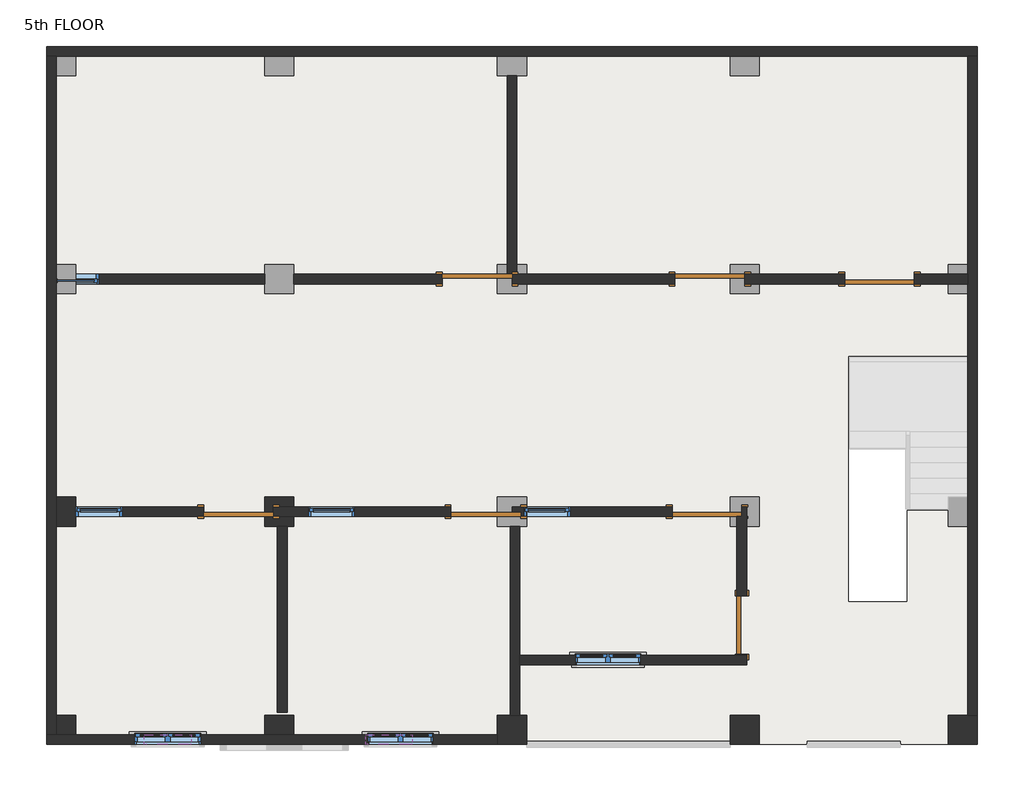
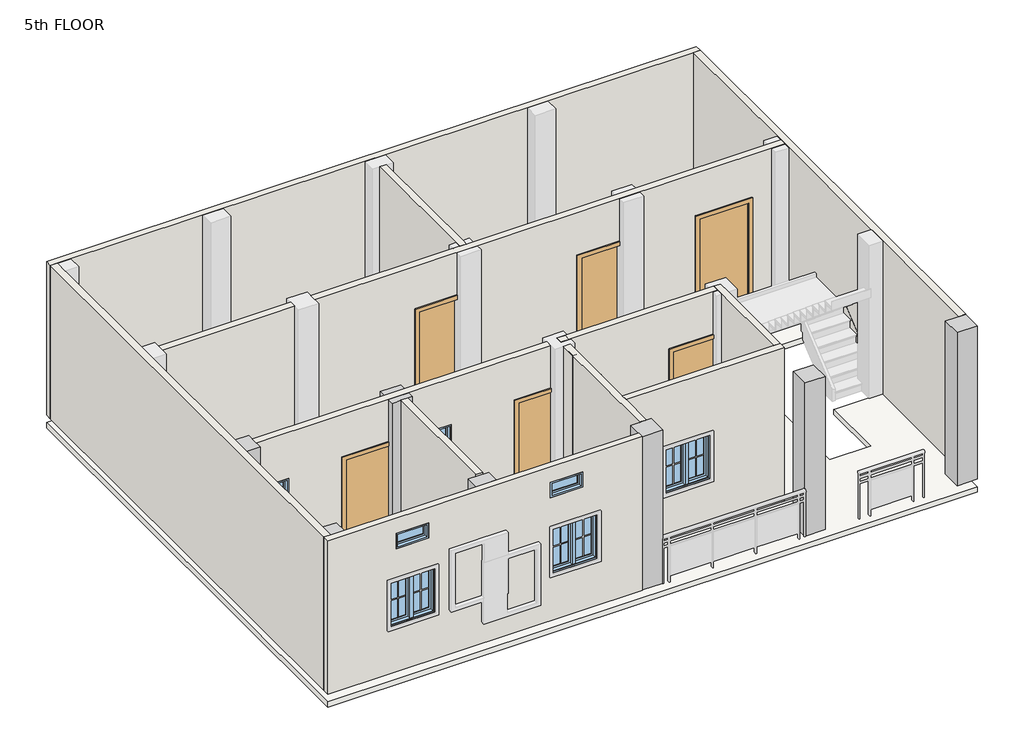
# One storey, part 1 of 2: 15 walls, 9 windows, 7 columns, 7 doors, 1 slab.
"""IFC4 building model written with IfcOpenShell, lengths in millimetres."""

from ifc_helpers import new_model, si_unit, frame, origin, place, context, project, spatial, polyline, outline, extrude, faceted_brep, transform, mapped, element, save
from components import door_e00f436c, door_a1797ceb, window_4c2727af, window_0bf3737e, window_78893e6c, window_0d9958e7

model = new_model("IFC4")

# Units and contexts
model_context = context("Model", 3, world=origin())
ifc_project = project(units=[si_unit("LENGTHUNIT", "METRE", prefix="MILLI")], contexts=[model_context])

# Site, building, storey
site = spatial("IfcSite", under=ifc_project)
building = spatial("IfcBuilding", under=site)
storey = spatial("IfcBuildingStorey", under=building, Name="5th FLOOR", Elevation=15087.6)

# Columns
placement = place(None, origin())
element("IfcColumn", 1, ObjectType="column family : column family", at=placement, inside=storey, context=model_context, shape_type="Brep", body=[
    faceted_brep([(-12576.097125, 2486.2065522, 15092.6), (-12957.097125, 2486.2065522, 15092.6), (-12957.097125, 2867.2065522, 15092.6), (-12576.097125, 2867.2065522, 15092.6), (-12576.097125, 2740.2065522, 15092.6), (-12842.797125, 2740.2065522, 15092.6), (-12842.797125, 2613.2065522, 15092.6), (-12576.097125, 2613.2065522, 15092.6), (-12576.097125, 2486.2065522, 18130.6), (-12576.097125, 2613.2065522, 18130.6), (-12957.097125, 2486.2065522, 18130.6), (-12957.097125, 2613.2065522, 18130.6), (-12957.097125, 2613.2065522, 17221.2), (-12957.097125, 2740.2065522, 17221.2), (-12957.097125, 2740.2065522, 18130.6), (-12957.097125, 2867.2065522, 18130.6), (-12576.097125, 2867.2065522, 18130.6), (-12842.797125, 2613.2065522, 17221.2), (-12842.797125, 2740.2065522, 17221.2), (-12576.097125, 2740.2065522, 18130.6)], [[[0, 1, 2, 3, 4, 5, 6, 7]], [[8, 0, 7, 9]], [[1, 0, 8, 10]], [[2, 1, 10, 11, 12, 13, 14, 15]], [[3, 2, 15, 16]], [[10, 8, 9, 11]], [[6, 17, 12, 11, 9, 7]], [[13, 18, 5, 4, 19, 14]], [[3, 16, 19, 4]], [[16, 15, 14, 19]], [[17, 18, 13, 12]], [[18, 17, 6, 5]]]),
])
element("IfcColumn", 2, ObjectType="column family : column family", at=placement, inside=storey, context=model_context, shape_type="SweptSolid", body=[
    extrude(outline(polyline([(-15433.597125, 2867.2065522), (-15433.597125, 2486.2065522), (-15687.597125, 2486.2065522), (-15687.597125, 2867.2065522), (-15433.597125, 2867.2065522)])), frame((0.0, 0.0, 15092.6), z_axis=(0.0, 0.0, 1.0), x_axis=(1.0, 0.0, 0.0)), (0.0, 0.0, 1.0), 3038.0),
])
element("IfcColumn", 3, ObjectType="column family : column family", at=placement, inside=storey, context=model_context, shape_type="SweptSolid", body=[
    extrude(outline(polyline([(-15433.597125, 9.7065522), (-15433.597125, -244.2934478), (-15687.597125, -244.2934478), (-15687.597125, 9.7065522), (-15433.597125, 9.7065522)])), frame((0.0, 0.0, 15092.6), z_axis=(0.0, 0.0, 1.0), x_axis=(1.0, 0.0, 0.0)), (0.0, 0.0, 1.0), 3038.0),
])
element("IfcColumn", 4, ObjectType="column family : column family", at=placement, inside=storey, context=model_context, shape_type="SweptSolid", body=[
    extrude(outline(polyline([(-3622.597125, 9.7065522), (-3622.597125, -371.2934478), (-4003.597125, -371.2934478), (-4003.597125, 9.7065522), (-3622.597125, 9.7065522)])), frame((0.0, 0.0, 15092.6), z_axis=(0.0, 0.0, 1.0), x_axis=(1.0, 0.0, 0.0)), (0.0, 0.0, 1.0), 3038.0),
])
element("IfcColumn", 5, ObjectType="column family : column family", at=placement, inside=storey, context=model_context, shape_type="SweptSolid", body=[
    extrude(outline(polyline([(-6480.097125, 9.7065522), (-6480.097125, -371.2934478), (-6861.097125, -371.2934478), (-6861.097125, 9.7065522), (-6480.097125, 9.7065522)])), frame((0.0, 0.0, 15092.6), z_axis=(0.0, 0.0, 1.0), x_axis=(1.0, 0.0, 0.0)), (0.0, 0.0, 1.0), 3038.0),
])
element("IfcColumn", 6, ObjectType="column family : column family", at=placement, inside=storey, context=model_context, shape_type="SweptSolid", body=[
    extrude(outline(polyline([(-9528.097125, 9.7065522), (-9528.097125, -371.2934478), (-9909.097125, -371.2934478), (-9909.097125, 9.7065522), (-9528.097125, 9.7065522)])), frame((0.0, 0.0, 15092.6), z_axis=(0.0, 0.0, 1.0), x_axis=(1.0, 0.0, 0.0)), (0.0, 0.0, 1.0), 3038.0),
])
element("IfcColumn", 7, ObjectType="column family : column family", at=placement, inside=storey, context=model_context, shape_type="SweptSolid", body=[
    extrude(outline(polyline([(-12957.097125, 9.7065522), (-12576.097125, 9.7065522), (-12576.097125, -244.2934478), (-12957.097125, -244.2934478), (-12957.097125, 9.7065522)])), frame((0.0, 0.0, 15092.6), z_axis=(0.0, 0.0, 1.0), x_axis=(1.0, 0.0, 0.0)), (0.0, 0.0, 1.0), 3038.0),
])

# Doors
door_shape = door_e00f436c(model_context)
element("IfcDoor", 8, ObjectType="Single-Flush : 30\" x 80\"", at=placement, inside=storey, context=model_context, shape_type="MappedRepresentation", body=[
    mapped(door_shape, transform((-6708.697125, 1190.8065522, 15087.6), x_axis=(0.0, -1.0, 0.0), y_axis=(1.0, 0.0, 0.0), z_axis=(0.0, 0.0, 1.0))),
])
door_2_shape = door_a1797ceb(model_context)
element("IfcDoor", 9, ObjectType="Single-Flush : 36\" x 84\"", at=placement, inside=storey, context=model_context, shape_type="MappedRepresentation", body=[
    mapped(door_2_shape, transform((-10175.797125, 5724.7065522, 15087.6), x_axis=(1.0, 0.0, 0.0), y_axis=(0.0, 1.0, 0.0), z_axis=(0.0, 0.0, 1.0))),
])
element("IfcDoor", 10, ObjectType="Single-Flush : 36\" x 84\"", at=placement, inside=storey, context=model_context, shape_type="MappedRepresentation", body=[
    mapped(door_2_shape, transform((-10061.497125, 2676.7065522, 15087.6), x_axis=(-1.0, 0.0, 0.0), y_axis=(0.0, -1.0, 0.0), z_axis=(0.0, 0.0, 1.0))),
])
element("IfcDoor", 11, ObjectType="Single-Flush : 36\" x 84\"", at=placement, inside=storey, context=model_context, shape_type="MappedRepresentation", body=[
    mapped(door_2_shape, transform((-13299.997125, 2676.7065522, 15087.6), x_axis=(-1.0, 0.0, 0.0), y_axis=(0.0, -1.0, 0.0), z_axis=(0.0, 0.0, 1.0))),
])
element("IfcDoor", 12, ObjectType="Single-Flush : 36\" x 84\"", at=placement, inside=storey, context=model_context, shape_type="MappedRepresentation", body=[
    mapped(door_2_shape, transform((-7127.797125, 5724.7065522, 15087.6), x_axis=(1.0, 0.0, 0.0), y_axis=(0.0, 1.0, 0.0), z_axis=(0.0, 0.0, 1.0))),
])
element("IfcDoor", 13, ObjectType="Single-Flush : 36\" x 84\"", at=placement, inside=storey, context=model_context, shape_type="MappedRepresentation", body=[
    mapped(door_2_shape, transform((-7165.897125, 2676.7065522, 15087.6), x_axis=(-1.0, 0.0, 0.0), y_axis=(0.0, -1.0, 0.0), z_axis=(0.0, 0.0, 1.0))),
])
element("IfcDoor", 14, ObjectType="Single-Flush : 36\" x 84\"", at=placement, inside=storey, context=model_context, shape_type="MappedRepresentation", body=[
    mapped(door_2_shape, transform((-4905.297125, 5724.7065522, 15087.6), x_axis=(-1.0, 0.0, 0.0), y_axis=(0.0, -1.0, 0.0), z_axis=(0.0, 0.0, 1.0))),
])

# Slab
element("IfcSlab", 15, ObjectType="Generic - 4\"", at=placement, inside=storey, context=model_context, shape_type="SweptSolid", body=[
    extrude(outline(polyline([(-3622.597125, 8772.7065522), (-3622.597125, -371.2934478), (-15814.597125, -371.2934478), (-15814.597125, 8772.7065522), (-3622.597125, 8772.7065522)]), holes=[polyline([(-3734.357125, 4711.0719226), (-5310.2646464, 4711.0719226), (-5310.2646464, 1502.3126957), (-4547.7736682, 1502.3126957), (-4547.7736682, 2699.911213), (-3734.357125, 2699.911213), (-3734.357125, 4711.0719226)])]), frame((0.0, 0.0, 14833.6), z_axis=(0.0, 0.0, 1.0), x_axis=(1.0, 0.0, 0.0)), (0.0, 0.0, 1.0), 101.6),
])

# Walls
element("IfcWall", 16, ObjectType="Generic - 5\"", at=placement, inside=storey, context=model_context, shape_type="Brep", body=[
    faceted_brep([(-15814.597125, 8645.7065522, 15087.6), (-15687.597125, 8645.7065522, 15087.6), (-3749.597125, 8645.7065522, 15087.6), (-3622.597125, 8645.7065522, 15087.6), (-3622.597125, 8645.7065522, 18135.6), (-3749.597125, 8645.7065522, 18135.6), (-15687.597125, 8645.7065522, 18135.6), (-15814.597125, 8645.7065522, 18135.6), (-15814.597125, 8772.7065522, 15087.6), (-15814.597125, 8772.7065522, 18135.6), (-3622.597125, 8772.7065522, 18135.6), (-3622.597125, 8772.7065522, 15087.6)], [[[0, 1, 2, 3, 4, 5, 6, 7]], [[8, 9, 10, 11]], [[3, 2, 1, 0, 8, 11]], [[7, 6, 5, 4, 10, 9]], [[4, 3, 11, 10]], [[0, 7, 9, 8]]]),
])
element("IfcWall", 17, ObjectType="Generic - 5\"", at=placement, inside=storey, context=model_context, shape_type="Brep", body=[
    faceted_brep([(-3749.597125, 8645.7065522, 15087.6), (-3749.597125, 5788.2065522, 15087.6), (-3749.597125, 5661.2065522, 15087.6), (-3749.597125, 9.7065522, 15087.6), (-3749.597125, 9.7065522, 18135.6), (-3749.597125, 5661.2065522, 18135.6), (-3749.597125, 5788.2065522, 18135.6), (-3749.597125, 8645.7065522, 18135.6), (-3622.597125, 8645.7065522, 15087.6), (-3622.597125, 8645.7065522, 18135.6), (-3622.597125, 9.7065522, 18135.6), (-3622.597125, 9.7065522, 18130.6), (-3622.597125, 9.7065522, 15092.6), (-3622.597125, 9.7065522, 15087.6)], [[[0, 1, 2, 3, 4, 5, 6, 7]], [[8, 9, 10, 11, 12, 13]], [[3, 2, 1, 0, 8, 13]], [[4, 3, 13, 12, 11, 10]], [[7, 6, 5, 4, 10, 9]], [[0, 7, 9, 8]]]),
])
element("IfcWall", 18, ObjectType="Generic - 5\"", at=placement, inside=storey, context=model_context, shape_type="Brep", body=[
    faceted_brep([(-9909.097125, -244.2934478, 15087.6), (-15687.597125, -244.2934478, 15087.6), (-15814.597125, -244.2934478, 15087.6), (-15814.597125, -244.2934478, 18135.6), (-15687.597125, -244.2934478, 18135.6), (-9909.097125, -244.2934478, 18135.6), (-13795.297125, -244.2934478, 16916.4), (-14658.897125, -244.2934478, 16916.4), (-14658.897125, -244.2934478, 16002.0), (-13795.297125, -244.2934478, 16002.0), (-10747.297125, -244.2934478, 16916.4), (-11610.897125, -244.2934478, 16916.4), (-11610.897125, -244.2934478, 16002.0), (-10747.297125, -244.2934478, 16002.0), (-13922.297125, -244.2934478, 17830.8), (-14531.897125, -244.2934478, 17830.8), (-14531.897125, -244.2934478, 17526.0), (-13922.297125, -244.2934478, 17526.0), (-11026.697125, -244.2934478, 17830.8), (-11636.297125, -244.2934478, 17830.8), (-11636.297125, -244.2934478, 17526.0), (-11026.697125, -244.2934478, 17526.0), (-9909.097125, -371.2934478, 15087.6), (-9909.097125, -371.2934478, 15092.6), (-9909.097125, -371.2934478, 18130.6), (-9909.097125, -371.2934478, 18135.6), (-15814.597125, -371.2934478, 18135.6), (-15814.597125, -371.2934478, 15087.6), (-13795.297125, -371.2934478, 16916.4), (-13795.297125, -371.2934478, 16002.0), (-14658.897125, -371.2934478, 16002.0), (-14658.897125, -371.2934478, 16916.4), (-10747.297125, -371.2934478, 16916.4), (-10747.297125, -371.2934478, 16002.0), (-11610.897125, -371.2934478, 16002.0), (-11610.897125, -371.2934478, 16916.4), (-13922.297125, -371.2934478, 17830.8), (-13922.297125, -371.2934478, 17526.0), (-14531.897125, -371.2934478, 17526.0), (-14531.897125, -371.2934478, 17830.8), (-11026.697125, -371.2934478, 17830.8), (-11026.697125, -371.2934478, 17526.0), (-11636.297125, -371.2934478, 17526.0), (-11636.297125, -371.2934478, 17830.8)], [[[0, 1, 2, 3, 4, 5], [6, 7, 8, 9], [10, 11, 12, 13], [14, 15, 16, 17], [18, 19, 20, 21]], [[22, 23, 24, 25, 26, 27], [28, 29, 30, 31], [32, 33, 34, 35], [36, 37, 38, 39], [40, 41, 42, 43]], [[2, 1, 0, 22, 27]], [[5, 4, 3, 26, 25]], [[0, 5, 25, 24, 23, 22]], [[3, 2, 27, 26]], [[29, 28, 6, 9]], [[30, 29, 9, 8]], [[31, 30, 8, 7]], [[28, 31, 7, 6]], [[33, 32, 10, 13]], [[34, 33, 13, 12]], [[35, 34, 12, 11]], [[32, 35, 11, 10]], [[37, 36, 14, 17]], [[38, 37, 17, 16]], [[39, 38, 16, 15]], [[36, 39, 15, 14]], [[41, 40, 18, 21]], [[42, 41, 21, 20]], [[43, 42, 20, 19]], [[40, 43, 19, 18]]]),
])
element("IfcWall", 19, ObjectType="Generic - 5\"", at=placement, inside=storey, context=model_context, shape_type="Brep", body=[
    faceted_brep([(-15687.597125, -244.2934478, 15087.6), (-15687.597125, 8645.7065522, 15087.6), (-15687.597125, 8645.7065522, 15092.6), (-15687.597125, 8645.7065522, 18130.6), (-15687.597125, 8645.7065522, 18135.6), (-15687.597125, -244.2934478, 18135.6), (-15687.597125, -244.2934478, 18130.6), (-15687.597125, -244.2934478, 15092.6), (-15814.597125, -244.2934478, 15087.6), (-15814.597125, -244.2934478, 18135.6), (-15814.597125, 8645.7065522, 18135.6), (-15814.597125, 8645.7065522, 15087.6)], [[[0, 1, 2, 3, 4, 5, 6, 7]], [[8, 9, 10, 11]], [[1, 0, 8, 11]], [[5, 4, 10, 9]], [[4, 3, 2, 1, 11, 10]], [[0, 7, 6, 5, 9, 8]]]),
])
element("IfcWall", 20, ObjectType="Generic - 5\"", at=placement, inside=storey, context=model_context, shape_type="SweptSolid", body=[
    extrude(outline(polyline([(15087.6, -15433.597125), (15087.6, -12957.097125), (18135.6, -12957.097125), (18135.6, -15433.597125), (17221.2, -15433.597125), (17221.2, -15128.797125), (15392.4, -15128.797125), (15392.4, -15433.597125), (15087.6, -15433.597125)])), frame((0.0, 5661.2065522, 0.0), z_axis=(0.0, 1.0, 0.0), x_axis=(0.0, 0.0, 1.0)), (0.0, 0.0, 1.0), 127.0),
])
element("IfcWall", 21, ObjectType="Generic - 5\"", at=placement, inside=storey, context=model_context, shape_type="Brep", body=[
    faceted_brep([(-9782.097125, 8391.7065522, 15087.6), (-9782.097125, 5788.2065522, 15087.6), (-9782.097125, 5788.2065522, 15092.6), (-9782.097125, 5788.2065522, 17221.2), (-9782.097125, 5788.2065522, 18130.6), (-9782.097125, 5788.2065522, 18135.6), (-9782.097125, 8391.7065522, 18135.6), (-9655.097125, 8391.7065522, 15087.6), (-9655.097125, 8391.7065522, 18135.6), (-9655.097125, 5788.2065522, 18135.6), (-9655.097125, 5788.2065522, 18130.6), (-9655.097125, 5788.2065522, 15092.6), (-9655.097125, 5788.2065522, 15087.6), (-9718.597125, 5788.2065522, 15087.6)], [[[0, 1, 2, 3, 4, 5, 6]], [[7, 8, 9, 10, 11, 12]], [[1, 0, 7, 12, 13]], [[6, 5, 9, 8]], [[0, 6, 8, 7]], [[5, 4, 3, 2, 1, 13, 12, 11, 10, 9]]]),
])
element("IfcWall", 22, ObjectType="Generic - 5\"", at=placement, inside=storey, context=model_context, shape_type="Brep", body=[
    faceted_brep([(-6670.597125, 5661.2065522, 15087.6), (-5362.497125, 5661.2065522, 15087.6), (-5362.497125, 5661.2065522, 17221.2), (-4448.097125, 5661.2065522, 17221.2), (-4448.097125, 5661.2065522, 15087.6), (-3749.597125, 5661.2065522, 15087.6), (-3749.597125, 5661.2065522, 15092.6), (-3749.597125, 5661.2065522, 18130.6), (-3749.597125, 5661.2065522, 18135.6), (-12576.097125, 5661.2065522, 18135.6), (-12576.097125, 5661.2065522, 15087.6), (-10632.997125, 5661.2065522, 15087.6), (-10632.997125, 5661.2065522, 17221.2), (-9909.097125, 5661.2065522, 17221.2), (-9718.597125, 5661.2065522, 17221.2), (-9718.597125, 5661.2065522, 15092.6), (-9718.597125, 5661.2065522, 15087.6), (-7584.997125, 5661.2065522, 15087.6), (-7584.997125, 5661.2065522, 17221.2), (-6861.097125, 5661.2065522, 17221.2), (-6670.597125, 5661.2065522, 17221.2), (-6670.597125, 5661.2065522, 15092.6), (-5362.497125, 5788.2065522, 17221.2), (-5362.497125, 5788.2065522, 15087.6), (-6670.597125, 5788.2065522, 15087.6), (-6670.597125, 5788.2065522, 15092.6), (-6670.597125, 5788.2065522, 17221.2), (-6861.097125, 5788.2065522, 17221.2), (-7584.997125, 5788.2065522, 17221.2), (-7584.997125, 5788.2065522, 15087.6), (-9655.097125, 5788.2065522, 15087.6), (-9718.597125, 5788.2065522, 15087.6), (-9718.597125, 5788.2065522, 15092.6), (-9718.597125, 5788.2065522, 17221.2), (-9782.097125, 5788.2065522, 17221.2), (-9909.097125, 5788.2065522, 17221.2), (-10632.997125, 5788.2065522, 17221.2), (-10632.997125, 5788.2065522, 15087.6), (-12576.097125, 5788.2065522, 15087.6), (-12576.097125, 5788.2065522, 18135.6), (-9782.097125, 5788.2065522, 18135.6), (-9655.097125, 5788.2065522, 18135.6), (-3749.597125, 5788.2065522, 18135.6), (-3749.597125, 5788.2065522, 18130.6), (-3749.597125, 5788.2065522, 15092.6), (-3749.597125, 5788.2065522, 15087.6), (-4448.097125, 5788.2065522, 15087.6), (-4448.097125, 5788.2065522, 17221.2)], [[[0, 1, 2, 3, 4, 5, 6, 7, 8, 9, 10, 11, 12, 13, 14, 15, 16, 17, 18, 19, 20, 21]], [[22, 23, 24, 25, 26, 27, 28, 29, 30, 31, 32, 33, 34, 35, 36, 37, 38, 39, 40, 41, 42, 43, 44, 45, 46, 47]], [[11, 10, 38, 37]], [[17, 16, 31, 30, 29]], [[46, 45, 5, 4]], [[24, 23, 1, 0]], [[9, 8, 42, 41, 40, 39]], [[10, 9, 39, 38]], [[8, 7, 6, 5, 45, 44, 43, 42]], [[33, 32, 31, 16, 15, 14]], [[36, 35, 34, 33, 14, 13, 12]], [[37, 36, 12, 11]], [[26, 25, 24, 0, 21, 20]], [[28, 27, 26, 20, 19, 18]], [[29, 28, 18, 17]], [[2, 1, 23, 22]], [[3, 2, 22, 47]], [[4, 3, 47, 46]]]),
])
element("IfcWall", 23, ObjectType="Generic - 5\"", at=placement, inside=storey, context=model_context, shape_type="Brep", body=[
    faceted_brep([(-14823.997125, 2613.2065522, 15392.4), (-15433.597125, 2613.2065522, 15392.4), (-15433.597125, 2613.2065522, 15087.6), (-13757.197125, 2613.2065522, 15087.6), (-13757.197125, 2613.2065522, 17221.2), (-12957.097125, 2613.2065522, 17221.2), (-12842.797125, 2613.2065522, 17221.2), (-12842.797125, 2613.2065522, 15092.6), (-12842.797125, 2613.2065522, 15087.6), (-10518.697125, 2613.2065522, 15087.6), (-10518.697125, 2613.2065522, 17221.2), (-9909.097125, 2613.2065522, 17221.2), (-9909.097125, 2613.2065522, 18135.6), (-15433.597125, 2613.2065522, 18135.6), (-15433.597125, 2613.2065522, 17221.2), (-14823.997125, 2613.2065522, 17221.2), (-12385.597125, 2613.2065522, 17221.2), (-11775.997125, 2613.2065522, 17221.2), (-11775.997125, 2613.2065522, 15392.4), (-12385.597125, 2613.2065522, 15392.4), (-15433.597125, 2740.2065522, 15087.6), (-15433.597125, 2740.2065522, 15392.4), (-14823.997125, 2740.2065522, 15392.4), (-14823.997125, 2740.2065522, 17221.2), (-15433.597125, 2740.2065522, 17221.2), (-15433.597125, 2740.2065522, 18135.6), (-9909.097125, 2740.2065522, 18135.6), (-9909.097125, 2740.2065522, 17221.2), (-10518.697125, 2740.2065522, 17221.2), (-10518.697125, 2740.2065522, 15087.6), (-12842.797125, 2740.2065522, 15087.6), (-12842.797125, 2740.2065522, 15092.6), (-12842.797125, 2740.2065522, 17221.2), (-12957.097125, 2740.2065522, 17221.2), (-13757.197125, 2740.2065522, 17221.2), (-13757.197125, 2740.2065522, 15087.6), (-12385.597125, 2740.2065522, 17221.2), (-12385.597125, 2740.2065522, 15392.4), (-11775.997125, 2740.2065522, 15392.4), (-11775.997125, 2740.2065522, 17221.2)], [[[0, 1, 2, 3, 4, 5, 6, 7, 8, 9, 10, 11, 12, 13, 14, 15], [16, 17, 18, 19]], [[20, 21, 22, 23, 24, 25, 26, 27, 28, 29, 30, 31, 32, 33, 34, 35], [36, 37, 38, 39]], [[30, 29, 9, 8]], [[20, 35, 3, 2]], [[26, 12, 11, 27]], [[13, 12, 26, 25]], [[14, 13, 25, 24]], [[2, 1, 21, 20]], [[28, 10, 9, 29]], [[10, 28, 27, 11]], [[4, 3, 35, 34]], [[6, 5, 4, 34, 33, 32]], [[8, 7, 6, 32, 31, 30]], [[22, 21, 1, 0]], [[23, 22, 0, 15]], [[24, 23, 15, 14]], [[37, 36, 16, 19]], [[38, 37, 19, 18]], [[39, 38, 18, 17]], [[36, 39, 17, 16]]]),
])
element("IfcWall", 24, ObjectType="Generic - 5\"", at=placement, inside=storey, context=model_context, shape_type="Brep", body=[
    faceted_brep([(-9616.997125, 9.7065522, 15087.6), (-9616.997125, 670.1065522, 15087.6), (-9616.997125, 797.1065522, 15087.6), (-9616.997125, 2486.2065522, 15087.6), (-9616.997125, 2486.2065522, 18135.6), (-9616.997125, 797.1065522, 18135.6), (-9616.997125, 670.1065522, 18135.6), (-9616.997125, 9.7065522, 18135.6), (-9743.997125, 9.7065522, 15087.6), (-9743.997125, 9.7065522, 18135.6), (-9743.997125, 2486.2065522, 18135.6), (-9743.997125, 2486.2065522, 15087.6)], [[[0, 1, 2, 3, 4, 5, 6, 7]], [[8, 9, 10, 11]], [[3, 2, 1, 0, 8, 11]], [[4, 3, 11, 10]], [[7, 6, 5, 4, 10, 9]], [[0, 7, 9, 8]]]),
])
element("IfcWall", 25, ObjectType="Generic - 5\"", at=placement, inside=storey, context=model_context, shape_type="SweptSolid", body=[
    extrude(outline(polyline([(-9743.997125, 2181.4065522), (-9743.997125, 2486.2065522), (-9616.997125, 2486.2065522), (-9616.997125, 2181.4065522), (-9743.997125, 2181.4065522)])), frame((0.0, 0.0, 15087.6), z_axis=(0.0, 0.0, 1.0), x_axis=(1.0, 0.0, 0.0)), (0.0, 0.0, 1.0), 3048.0),
])
element("IfcWall", 26, ObjectType="Generic - 5\"", at=placement, inside=storey, context=model_context, shape_type="Brep", body=[
    faceted_brep([(-6772.197125, 2613.2065522, 18135.6), (-9718.597125, 2613.2065522, 18135.6), (-9718.597125, 2613.2065522, 18130.6), (-9718.597125, 2613.2065522, 15092.6), (-9718.597125, 2613.2065522, 15087.6), (-7623.097125, 2613.2065522, 15087.6), (-7623.097125, 2613.2065522, 17221.2), (-6861.097125, 2613.2065522, 17221.2), (-6772.197125, 2613.2065522, 17221.2), (-6772.197125, 2613.2065522, 18130.6), (-9566.197125, 2613.2065522, 17221.2), (-9528.097125, 2613.2065522, 17221.2), (-8956.597125, 2613.2065522, 17221.2), (-8956.597125, 2613.2065522, 15392.4), (-9528.097125, 2613.2065522, 15392.4), (-9566.197125, 2613.2065522, 15392.4), (-9718.597125, 2740.2065522, 18135.6), (-6772.197125, 2740.2065522, 18135.6), (-6772.197125, 2740.2065522, 17221.2), (-6861.097125, 2740.2065522, 17221.2), (-7623.097125, 2740.2065522, 17221.2), (-7623.097125, 2740.2065522, 15087.6), (-9718.597125, 2740.2065522, 15087.6), (-9718.597125, 2740.2065522, 15092.6), (-9718.597125, 2740.2065522, 18130.6), (-9566.197125, 2740.2065522, 17221.2), (-9566.197125, 2740.2065522, 15392.4), (-9528.097125, 2740.2065522, 15392.4), (-8956.597125, 2740.2065522, 15392.4), (-8956.597125, 2740.2065522, 17221.2), (-9528.097125, 2740.2065522, 17221.2)], [[[0, 1, 2, 3, 4, 5, 6, 7, 8, 9], [10, 11, 12, 13, 14, 15]], [[16, 17, 18, 19, 20, 21, 22, 23, 24], [25, 26, 27, 28, 29, 30]], [[4, 22, 21, 5]], [[1, 0, 17, 16]], [[4, 3, 2, 1, 16, 24, 23, 22]], [[26, 25, 10, 15]], [[28, 27, 26, 15, 14, 13]], [[29, 28, 13, 12]], [[25, 30, 29, 12, 11, 10]], [[20, 6, 5, 21]], [[6, 20, 19, 18, 8, 7]], [[17, 0, 9, 8, 18]]]),
])
element("IfcWall", 27, ObjectType="Generic - 5\"", at=placement, inside=storey, context=model_context, shape_type="Brep", body=[
    faceted_brep([(-6645.197125, 797.1065522, 15087.6), (-6645.197125, 809.8065522, 15087.6), (-6645.197125, 809.8065522, 17119.6), (-6645.197125, 1571.8065522, 17119.6), (-6645.197125, 1571.8065522, 15087.6), (-6645.197125, 2740.2065522, 15087.6), (-6645.197125, 2740.2065522, 15092.6), (-6645.197125, 2740.2065522, 18130.6), (-6645.197125, 2740.2065522, 18135.6), (-6645.197125, 797.1065522, 18135.6), (-6772.197125, 809.8065522, 17119.6), (-6772.197125, 809.8065522, 15087.6), (-6772.197125, 797.1065522, 15087.6), (-6772.197125, 797.1065522, 18135.6), (-6772.197125, 2613.2065522, 18135.6), (-6772.197125, 2740.2065522, 18135.6), (-6772.197125, 2740.2065522, 17221.2), (-6772.197125, 2613.2065522, 17221.2), (-6772.197125, 2613.2065522, 15092.6), (-6772.197125, 2613.2065522, 15087.6), (-6772.197125, 1571.8065522, 15087.6), (-6772.197125, 1571.8065522, 17119.6), (-6708.697125, 2613.2065522, 15087.6), (-6708.697125, 2740.2065522, 15087.6), (-6708.697125, 2613.2065522, 17221.2), (-6708.697125, 2613.2065522, 15092.6), (-6708.697125, 2740.2065522, 17221.2), (-6708.697125, 2740.2065522, 15092.6)], [[[0, 1, 2, 3, 4, 5, 6, 7, 8, 9]], [[10, 11, 12, 13, 14, 15, 16, 17, 18, 19, 20, 21]], [[20, 19, 22, 23, 5, 4]], [[12, 11, 1, 0]], [[9, 8, 15, 14, 13]], [[24, 25, 22, 19, 18, 17]], [[26, 24, 17, 16]], [[22, 25, 24, 26, 27, 23]], [[8, 7, 6, 5, 23, 27, 26, 16, 15]], [[0, 9, 13, 12]], [[2, 1, 11, 10]], [[3, 2, 10, 21]], [[4, 3, 21, 20]]]),
])
element("IfcWall", 28, ObjectType="Generic - 5\"", at=placement, inside=storey, context=model_context, shape_type="Brep", body=[
    faceted_brep([(-9718.597125, 2613.2065522, 15087.6), (-9566.197125, 2613.2065522, 15087.6), (-9566.197125, 2613.2065522, 15392.4), (-9566.197125, 2613.2065522, 17221.2), (-9566.197125, 2613.2065522, 18135.6), (-9718.597125, 2613.2065522, 18135.6), (-9718.597125, 2613.2065522, 18130.6), (-9718.597125, 2613.2065522, 15092.6), (-9718.597125, 2740.2065522, 15087.6), (-9718.597125, 2740.2065522, 15092.6), (-9718.597125, 2740.2065522, 18130.6), (-9718.597125, 2740.2065522, 18135.6), (-9566.197125, 2740.2065522, 18135.6), (-9566.197125, 2740.2065522, 17221.2), (-9566.197125, 2740.2065522, 15392.4), (-9566.197125, 2740.2065522, 15087.6)], [[[0, 1, 2, 3, 4, 5, 6, 7]], [[8, 9, 10, 11, 12, 13, 14, 15]], [[1, 0, 8, 15]], [[4, 3, 2, 1, 15, 14, 13, 12]], [[5, 4, 12, 11]], [[0, 7, 6, 5, 11, 10, 9, 8]]]),
])
element("IfcWall", 29, ObjectType="Generic - 5\"", at=placement, inside=storey, context=model_context, shape_type="SweptSolid", body=[
    extrude(outline(polyline([(-12791.997125, 47.8065522), (-12791.997125, 2486.2065522), (-12664.997125, 2486.2065522), (-12664.997125, 47.8065522), (-12791.997125, 47.8065522)])), frame((0.0, 0.0, 15087.6), z_axis=(0.0, 0.0, 1.0), x_axis=(1.0, 0.0, 0.0)), (0.0, 0.0, 1.0), 3048.0),
])
element("IfcWall", 30, ObjectType="Generic - 5\"", at=placement, inside=storey, context=model_context, shape_type="Brep", body=[
    faceted_brep([(-9616.997125, 670.1065522, 15087.6), (-6645.197125, 670.1065522, 15087.6), (-6645.197125, 670.1065522, 18135.6), (-9616.997125, 670.1065522, 18135.6), (-8029.497125, 670.1065522, 16916.4), (-8029.497125, 670.1065522, 16002.0), (-8893.097125, 670.1065522, 16002.0), (-8893.097125, 670.1065522, 16916.4), (-9616.997125, 797.1065522, 15087.6), (-9616.997125, 797.1065522, 18135.6), (-6772.197125, 797.1065522, 18135.6), (-6645.197125, 797.1065522, 18135.6), (-6645.197125, 797.1065522, 15087.6), (-6772.197125, 797.1065522, 15087.6), (-8029.497125, 797.1065522, 16916.4), (-8893.097125, 797.1065522, 16916.4), (-8893.097125, 797.1065522, 16002.0), (-8029.497125, 797.1065522, 16002.0)], [[[0, 1, 2, 3], [4, 5, 6, 7]], [[8, 9, 10, 11, 12, 13], [14, 15, 16, 17]], [[1, 0, 8, 13, 12]], [[3, 2, 11, 10, 9]], [[0, 3, 9, 8]], [[2, 1, 12, 11]], [[5, 4, 14, 17]], [[6, 5, 17, 16]], [[7, 6, 16, 15]], [[4, 7, 15, 14]]]),
])

# Windows
window_shape = window_4c2727af(model_context)
element("IfcWindow", 31, ObjectType="Fixed : 24\" x 12\"", at=placement, inside=storey, context=model_context, shape_type="MappedRepresentation", body=[
    mapped(window_shape, transform((-14188.997125, -307.7934478, 16611.6), x_axis=(1.0, 0.0, 0.0), y_axis=(0.0, 1.0, 0.0), z_axis=(0.0, 0.0, 1.0))),
])
element("IfcWindow", 32, ObjectType="Fixed : 24\" x 12\"", at=placement, inside=storey, context=model_context, shape_type="MappedRepresentation", body=[
    mapped(window_shape, transform((-11293.397125, -307.7934478, 16611.6), x_axis=(1.0, 0.0, 0.0), y_axis=(0.0, 1.0, 0.0), z_axis=(0.0, 0.0, 1.0))),
])
window_2_shape = window_0bf3737e(model_context)
element("IfcWindow", 33, ObjectType="Fixed : 24\" x 72\"", at=placement, inside=storey, context=model_context, shape_type="MappedRepresentation", body=[
    mapped(window_2_shape, transform((-15471.697125, 5724.7065522, 15087.6), x_axis=(-1.0, 0.0, 0.0), y_axis=(0.0, -1.0, 0.0), z_axis=(0.0, 0.0, 1.0))),
])
window_3_shape = window_78893e6c(model_context)
element("IfcWindow", 34, ObjectType="Fixed : 24\" x 72\"", at=placement, inside=storey, context=model_context, shape_type="MappedRepresentation", body=[
    mapped(window_3_shape, transform((-15166.897125, 2676.7065522, 15087.6), x_axis=(-1.0, 0.0, 0.0), y_axis=(0.0, -1.0, 0.0), z_axis=(0.0, 0.0, 1.0))),
])
element("IfcWindow", 35, ObjectType="Fixed : 24\" x 72\"", at=placement, inside=storey, context=model_context, shape_type="MappedRepresentation", body=[
    mapped(window_3_shape, transform((-12118.897125, 2676.7065522, 15087.6), x_axis=(-1.0, 0.0, 0.0), y_axis=(0.0, -1.0, 0.0), z_axis=(0.0, 0.0, 1.0))),
])
element("IfcWindow", 36, ObjectType="Fixed : 24\" x 72\"", at=placement, inside=storey, context=model_context, shape_type="MappedRepresentation", body=[
    mapped(window_3_shape, transform((-9299.497125, 2676.7065522, 15087.6), x_axis=(-1.0, 0.0, 0.0), y_axis=(0.0, -1.0, 0.0), z_axis=(0.0, 0.0, 1.0))),
])
window_4_shape = window_0d9958e7(model_context)
element("IfcWindow", 37, ObjectType="Window-Casement-Double : 34\" x 36\"", at=placement, inside=storey, context=model_context, shape_type="MappedRepresentation", body=[
    mapped(window_4_shape, transform((-14227.097125, -307.7934478, 15087.6), x_axis=(1.0, 0.0, 0.0), y_axis=(0.0, 1.0, 0.0), z_axis=(0.0, 0.0, 1.0))),
])
element("IfcWindow", 38, ObjectType="Window-Casement-Double : 34\" x 36\"", at=placement, inside=storey, context=model_context, shape_type="MappedRepresentation", body=[
    mapped(window_4_shape, transform((-11179.097125, -307.7934478, 15087.6), x_axis=(1.0, 0.0, 0.0), y_axis=(0.0, 1.0, 0.0), z_axis=(0.0, 0.0, 1.0))),
])
element("IfcWindow", 39, ObjectType="Window-Casement-Double : 34\" x 36\"", at=placement, inside=storey, context=model_context, shape_type="MappedRepresentation", body=[
    mapped(window_4_shape, transform((-8461.297125, 733.6065522, 15087.6), x_axis=(1.0, 0.0, 0.0), y_axis=(0.0, 1.0, 0.0), z_axis=(0.0, 0.0, 1.0))),
])

save(model, "model.ifc")

# Revit data of these elements
# Type "column family : column family"
#   w2 [instance default] = 0' - 9.88189"
#   w1 [instance default] = 0' - 9.01575"
#   Depth = 1' - 11.62205"
#   Width = 1' - 11.62205"
# Type "Single-Flush : 30\" x 80\""
#   Type Mark = "5"
#   Construction Type Id = "MDOOR"
#   Assembly Code = "C1020"
#   Analytic Construction = "Metal"
#   Thickness = 0' - 2"
#   Heat Transfer Coefficient (U) = 0.651978 BTU/(h·ft²·°F)
#   Height = 6' - 8"
#   Trim Projection Ext = 0' - 1"
#   Trim Projection Int = 0' - 1"
#   Trim Width = 0' - 3"
#   Width = 2' - 6"
#   Define Thermal Properties by = 1
#   Define Thermal Properties by = 1
#   Door Material = Door - Panel
#   Frame Material = Door - Frame
#   Visual Light Transmittance = 0
#   Solar Heat Gain Coefficient = 0
#   Function = (empty or 0)
#   Wall Closure = (empty or 0)
# Type "Single-Flush : 36\" x 84\""
#   Type Mark = "1"
#   Construction Type Id = "MDOOR"
#   Assembly Code = "C1020"
#   Analytic Construction = "Metal"
#   Thickness = 0' - 2"
#   Heat Transfer Coefficient (U) = 0.651978 BTU/(h·ft²·°F)
#   Height = 7' - 0"
#   Trim Projection Ext = 0' - 1"
#   Trim Projection Int = 0' - 1"
#   Trim Width = 0' - 3"
#   Width = 3' - 0"
#   Define Thermal Properties by = 1
#   Define Thermal Properties by = 1
#   Door Material = Door - Panel
#   Frame Material = Door - Frame
#   Visual Light Transmittance = 0
#   Solar Heat Gain Coefficient = 0
#   Function = (empty or 0)
#   Wall Closure = (empty or 0)
# Type "Generic - 4\""
#   Assembly Code = "B1010"
#   Function = 0
#   Layers, outside or top first: 0' - 4" no material (function 1)
# Type "Generic - 5\""
#   Assembly Code = "B2010"
#   Layers, outside or top first: 0' - 5" no material (function 1)
# Type "Fixed : 24\" x 12\""
#   Type Mark = "4"
#   Construction Type Id = "GSP4R"
#   Assembly Code = "B2020100"
#   Analytic Construction = "1/8 in Pilkington single glazing"
#   Visual Light Transmittance = 0.9
#   Solar Heat Gain Coefficient = 0.78
#   Heat Transfer Coefficient (U) = 0.6496 BTU/(h·ft²·°F)
#   Height = 1' - 0"
#   Default Sill Height = 3' - 0"
#   Width = 2' - 0"
#   Window Inset = 0' - 0 3/4"
#   Define Thermal Properties by = 1
#   Define Thermal Properties by = 1
#   Glass Pane Material = Glass
#   Sash Material = Sash
#   Wall Closure = (empty or 0)
# Type "Fixed : 24\" x 72\""
#   Type Mark = "7"
#   Construction Type Id = "GSP4R"
#   Assembly Code = "B2020100"
#   Analytic Construction = "1/8 in Pilkington single glazing"
#   Visual Light Transmittance = 0.9
#   Solar Heat Gain Coefficient = 0.78
#   Heat Transfer Coefficient (U) = 0.6496 BTU/(h·ft²·°F)
#   Height = 6' - 0"
#   Default Sill Height = 1' - 0"
#   Width = 2' - 0"
#   Window Inset = 0' - 0 3/4"
#   Define Thermal Properties by = 1
#   Define Thermal Properties by = 1
#   Glass Pane Material = Glass
#   Sash Material = Sash
#   Wall Closure = (empty or 0)
# Type "Window-Casement-Double : 34\" x 36\""
#   Type Mark = "14"
#   Fire Rating = "0.5h"
#   Assembly Code = "B2020100"
#   Analytic Construction = "Double glazing - domestic"
#   Frame Extension [instance default] = 0' - 0 1/4"
#   Window Inset [instance default] = 0' - 0"
#   Wall Thickness [instance default] = 0' - 6"
#   Interior Wall Closure [instance default] = 0' - 2 1/4"
#   Half Width = 1' - 5"
#   Visual Light Transmittance = 0.81
#   Thermal Resistance (R) = 1.8146 (h·ft²·°F)/BTU
#   Solar Heat Gain Coefficient = 0.76
#   Rough Width = 2' - 10 1/2"
#   Rough Height = 3' - 0 1/2"
#   Height = 3' - 0"
#   Heat Transfer Coefficient (U) = 0.5511 BTU/(h·ft²·°F)
#   Exterior Wall Closure [instance default] = 0' - 1 1/4"
#   Extension Jamb [instance default] = 0' - 2 1/4"
#   Default Sill Height = 3' - 0"
#   Width = 2' - 10"
#   Define Thermal Properties by = 0
#   Muntin Visibility = yes
#   Interior Trim Visibility [instance default] = yes
#   Exterior Trim Visibility [instance default] = yes
#   Extension Jamb Visibility [instance default] = yes
#   Interior Trim Material = Wood - Stained
#   Muntin Pattern = Muntin Pattern_2x2 : Muntin Pattern_2x2
#   Interior Trim = Trim-Window-Interior-Flat : Picture Frame
#   Interior Frame Material = Wood - Stained
#   Glass Panel Material = Glass
#   Exterior Trim Material = Clad - White
#   Exterior Trim = Trim-Window-Exterior-Flat : with Sill
#   Exterior Frame Material = Clad - White
#   Wall Closure = (empty or 0)
# Element 1 (IfcColumn, "column family : column family")
#   w2 = 1' - 3"
#   w1 = 1' - 3"
#   Phase Created = New Construction
#   Materials on its faces: "Default Wall", "inside wall"
# Element 2 (IfcColumn, "column family : column family")
#   w2 = 1' - 3"
#   w1 = 0' - 10"
#   Phase Created = New Construction
#   Materials on its faces: "inside wall", "Default Wall"
# Elements 3, 7 (IfcColumn, "column family : column family")
#   w2 = 1' - 3"
#   w1 = 1' - 3"
#   Phase Created = New Construction
#   Materials on its faces: "Default Wall"
# Element 4 (IfcColumn, "column family : column family")
#   w2 = 1' - 3"
#   w1 = 1' - 3"
#   Phase Created = New Construction
#   Materials on its faces: "Clad - White", "Default Wall"
# Element 5 (IfcColumn, "column family : column family")
#   w2 = 1' - 3"
#   w1 = 1' - 3"
#   Phase Created = New Construction
#   Materials on its faces: "out side wall"
# Element 6 (IfcColumn, "column family : column family")
#   w2 = 1' - 3"
#   w1 = 1' - 3"
#   Phase Created = New Construction
#   Materials on its faces: "out side wall", "Default Wall"
# Element 8 (IfcDoor, "Single-Flush : 30\" x 80\"")
#   Phase Created = New Construction
#   Materials on its faces: "Door - Frame", "Door - Panel"
# Elements 9, 10, 11, 12, 13, 14 (IfcDoor, "Single-Flush : 36\" x 84\"")
#   Phase Created = New Construction
#   Materials on its faces: "Door - Frame", "Door - Panel"
# Element 15 (IfcSlab, "Generic - 4\"")
#   Height Offset From Level = -0' - 6"
#   Phase Created = New Construction
#   Materials on its faces: "Default Floor", "Clad - White", "floor"
# Element 16 (IfcWall, "Generic - 5\"")
#   Top Offset = 0' - 0"
#   Base Offset = 0' - 0"
#   wall height = 10' - 0"
#   Phase Created = New Construction
#   Base Constraint = 5th FLOOR
#   Top Constraint = 6th FLOOR
#   Materials on its faces: "Default Wall", "Clad - White"
# Element 17 (IfcWall, "Generic - 5\"")
#   Top Offset = 0' - 0"
#   Base Offset = 0' - 0"
#   wall height = 10' - 0"
#   Phase Created = New Construction
#   Base Constraint = 5th FLOOR
#   Top Constraint = 6th FLOOR
#   Materials on its faces: "Default Wall", "grey", "Clad - White"
# Element 18 (IfcWall, "Generic - 5\"")
#   Top Offset = 0' - 0"
#   Base Offset = 0' - 0"
#   wall height = 10' - 0"
#   Phase Created = New Construction
#   Base Constraint = 5th FLOOR
#   Top Constraint = 6th FLOOR
#   Materials on its faces: "Default Wall", "out side wall", "Clad - White"
# Element 19 (IfcWall, "Generic - 5\"")
#   Top Offset = 0' - 0"
#   Base Offset = 0' - 0"
#   wall height = 10' - 0"
#   Phase Created = New Construction
#   Base Constraint = 5th FLOOR
#   Top Constraint = 6th FLOOR
#   Materials on its faces: "Default Wall", "inside wall", "Clad - White"
# Elements 20, 23, 26, 27 (IfcWall, "Generic - 5\"")
#   Top Offset = 0' - 0"
#   Base Offset = 0' - 0"
#   wall height = 10' - 0"
#   Phase Created = New Construction
#   Base Constraint = 5th FLOOR
#   Top Constraint = 6th FLOOR
#   Materials on its faces: "Default Wall", "inside wall"
# Elements 21, 25, 28, 29 (IfcWall, "Generic - 5\"")
#   Top Offset = 0' - 0"
#   Base Offset = 0' - 0"
#   wall height = 10' - 0"
#   Phase Created = New Construction
#   Base Constraint = 5th FLOOR
#   Top Constraint = 6th FLOOR
#   Materials on its faces: "Default Wall"
# Elements 22, 24 (IfcWall, "Generic - 5\"")
#   Top Offset = 0' - 0"
#   Base Offset = 0' - 0"
#   wall height = 10' - 0"
#   Phase Created = New Construction
#   Base Constraint = 5th FLOOR
#   Top Constraint = 6th FLOOR
#   Materials on its faces: "Default Wall", "grey"
# Element 30 (IfcWall, "Generic - 5\"")
#   Top Offset = 0' - 0"
#   Base Offset = 0' - 0"
#   wall height = 10' - 0"
#   Phase Created = New Construction
#   Base Constraint = 5th FLOOR
#   Top Constraint = 6th FLOOR
#   Materials on its faces: "Default Wall", "grey", "inside wall"
# Element 31 (IfcWindow, "Fixed : 24\" x 12\"")
#   Mark = "52"
#   Phase Created = New Construction
#   Materials on its faces: "Sash", "Glass"
# Element 32 (IfcWindow, "Fixed : 24\" x 12\"")
#   Mark = "53"
#   Phase Created = New Construction
#   Materials on its faces: "Sash", "Glass"
# Element 33 (IfcWindow, "Fixed : 24\" x 72\"")
#   Mark = "46"
#   Phase Created = New Construction
#   Materials on its faces: "Sash", "Glass"
# Element 34 (IfcWindow, "Fixed : 24\" x 72\"")
#   Mark = "47"
#   Phase Created = New Construction
#   Materials on its faces: "Sash", "Glass"
# Element 35 (IfcWindow, "Fixed : 24\" x 72\"")
#   Mark = "48"
#   Phase Created = New Construction
#   Materials on its faces: "Sash", "Glass"
# Element 36 (IfcWindow, "Fixed : 24\" x 72\"")
#   Mark = "49"
#   Phase Created = New Construction
#   Materials on its faces: "Sash", "Glass"
# Element 37 (IfcWindow, "Window-Casement-Double : 34\" x 36\"")
#   Mark = "50"
#   Window Inset = 0' - 0"
#   Interior Wall Closure = 0' - 2 1/4"
#   Frame Extension = 0' - 0 1/4"
#   Exterior Wall Closure = 0' - 1 1/4"
#   Interior Trim Visibility = yes
#   Exterior Trim Visibility = yes
#   Phase Created = New Construction
#   Materials on its faces: "Wood - Stained", "Glass", "Clad - White"
# Element 38 (IfcWindow, "Window-Casement-Double : 34\" x 36\"")
#   Mark = "51"
#   Window Inset = 0' - 0"
#   Interior Wall Closure = 0' - 2 1/4"
#   Frame Extension = 0' - 0 1/4"
#   Exterior Wall Closure = 0' - 1 1/4"
#   Interior Trim Visibility = yes
#   Exterior Trim Visibility = yes
#   Phase Created = New Construction
#   Materials on its faces: "Wood - Stained", "Glass", "Clad - White"
# Element 39 (IfcWindow, "Window-Casement-Double : 34\" x 36\"")
#   Mark = "54"
#   Window Inset = 0' - 0"
#   Interior Wall Closure = 0' - 2 1/4"
#   Frame Extension = 0' - 0 1/4"
#   Exterior Wall Closure = 0' - 1 1/4"
#   Interior Trim Visibility = yes
#   Exterior Trim Visibility = yes
#   Phase Created = New Construction
#   Materials on its faces: "Wood - Stained", "Glass", "Clad - White"
# Materials
#   "Door - Panel": class "Wood", colour RGB 210 159 95, transparency 0, Cost = 0
#   "Door - Frame": colour RGB 118 70 51, transparency 0, Cost = 0
#   "Glass": class "Glass", colour RGB 0 128 192, transparency 0.75, Description = "Soda Lime Glass", Cost = 0
#   "Sash": class "Wood", colour RGB 224 178 126, transparency 0, Cost = 0
#   "Wood - Stained": class "Wood", colour RGB 224 178 126, transparency 0, Cost = 0
#   "Clad - White": class "Wood", colour RGB 242 242 238, transparency 0, Cost = 0
#   "Default Wall": colour RGB 128 128 128, transparency 0, Cost = 0
#   "inside wall": class "Generic", colour RGB 199 224 95, transparency 0, Cost = 0
#   "out side wall": class "Generic", colour RGB 16 106 159, transparency 0, Cost = 0
#   "Default Floor": colour RGB 128 128 128, transparency 0, Cost = 0
#   "floor": class "Generic", colour RGB 255 255 255, transparency 0, Cost = 0
#   "grey": class "Generic", colour RGB 80 80 80, transparency 0, Cost = 0
